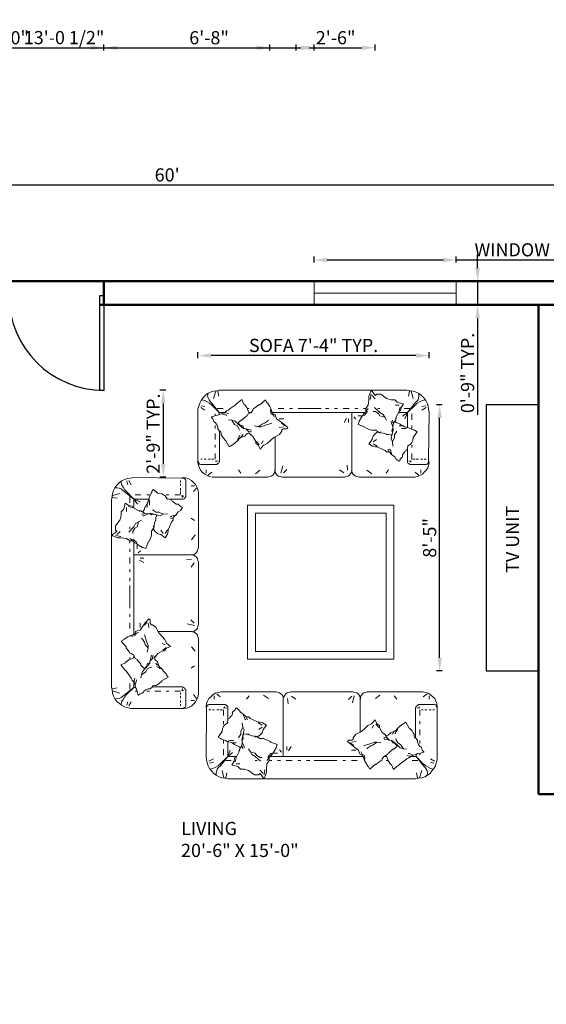
# Model space of a CAD drawing. Units: inches. Extents: x -46 to 764, y -530 to 112.
# Tile 4 of 5: x 307 to 507, y -262 to 112. Entities that reach past the tile are written whole.
import ezdxf

# ---------------------------------------------------------------- set-up
doc = ezdxf.new("R2010")
doc.units = ezdxf.units.IN
for name, color, linetype, lineweight in [('A-ANNO-DIMS', 2, 'Continuous', 18), ('A-AREA-IDEN', 7, 'Continuous', 18), ('A-DOOR', 3, 'Continuous', 25), ('A-FLOR-CASE', 32, 'Continuous', 25), ('A-GLAZ', 4, 'Continuous', 18), ('A-WALL', 7, 'Continuous', 50), ('furn', 28, 'Continuous', 18), ('txt', 167, 'Continuous', 18)]:
    doc.layers.add(name, color=color, linetype=linetype, lineweight=lineweight)
doc.styles.get("Standard").update_dxf_attribs({"font": 'arial.ttf'})
doc.dimstyles.new('ISO-25', dxfattribs={"dimtxt": 5, "dimasz": 5, "dimexe": 1.25, "dimexo": 0.625, "dimtad": 1, "dimlunit": 3, "dimtxsty": 'Standard', "dimcen": 2.5, "dimadec": 0, "dimazin": 0, "dimtfac": 1, "dimtmove": 0, "dimatfit": 3, "dimfxl": 1, "dimfxlon": 1, "dimarcsym": 0})

# ---------------------------------------------------------------- blocks, each defined once
blk = doc.blocks.new('*U2')
for p, q in [((0, 0), (0, -6)), ((40, 0), (40, -6))]:
    blk.add_line(p, q)
blk.add_lwpolyline([(0, 0), (0, 40), (1.75, 40), (1.75, 0)], close=True)
blk.add_arc((0, 0), 40, 0, 90)
blk = doc.blocks.new('sofa-36')
at = {"color": 0, "linetype": 'ByBlock'}
for p, q in [((-0.215, 0.805), (-0.2, 0.83)), ((-0.2, 0.83), (-0.215, 0.805)), ((-0.2, 0.83), (-0.18, 0.85)), ((-0.18, 0.85), (-0.2, 0.83)), ((-0.18, 0.85), (-0.16, 0.87)), ((-0.16, 0.87), (-0.18, 0.85)), ((-0.16, 0.87), (-0.135, 0.885)), ((-0.135, 0.885), (-0.16, 0.87)), ((-0.145, 0.825), (-0.145, 0.86)), ((-0.135, 0.885), (-0.105, 0.895)), ((-0.105, 0.895), (-0.135, 0.885)), ((-0.085, 0.85), (-0.12, 0.88)), ((-0.105, 0.895), (-0.08, 0.9)), ((-0.08, 0.9), (-0.105, 0.895)), ((-0.08, 0.9), (0.495, 0.9)), ((0.495, 0.9), (-0.08, 0.9)), ((0.19, 0.825), (0.215, 0.86)), ((0.415, 0.83), (0.365, 0.865)), ((0.495, 0.9), (0.515, 0.895)), ((0.515, 0.895), (0.495, 0.9)), ((0.515, 0.895), (0.53, 0.89)), ((0.53, 0.89), (0.515, 0.895)), ((0.53, 0.89), (0.545, 0.88)), ((0.545, 0.88), (0.53, 0.89)), ((0.545, 0.88), (0.56, 0.865)), ((0.56, 0.865), (0.545, 0.88)), ((0.56, 0.865), (0.57, 0.85)), ((0.57, 0.85), (0.56, 0.865)), ((0.57, 0.83), (0.575, 0.85)), ((0.57, 0.85), (0.57, 0.83)), ((0.57, 0.83), (0.57, 0.85)), ((0.57, 0.83), (0.575, 0.85)), ((0.57, 0.835), (0.57, 0.23)), ((0.57, 0.815), (0.57, 0.83)), ((0.57, 0.815), (0.57, 0.83)), ((0.575, 0.85), (0.585, 0.865)), ((0.575, 0.85), (0.585, 0.865)), ((0.585, 0.865), (0.595, 0.88)), ((0.585, 0.865), (0.595, 0.88)), ((0.595, 0.88), (0.61, 0.89)), ((0.595, 0.88), (0.61, 0.89)), ((0.61, 0.89), (0.63, 0.895)), ((0.61, 0.89), (0.63, 0.895)), ((0.615, 0.83), (0.62, 0.775)), ((0.63, 0.895), (0.645, 0.9)), ((0.63, 0.895), (0.645, 0.9)), ((0.645, 0.9), (0.87, 0.9)), ((0.87, 0.9), (0.645, 0.9)), ((0.655, 0.855), (0.7, 0.825)), ((0.87, 0.9), (1.29, 0.9)), ((1.29, 0.9), (0.87, 0.9)), ((1.28, 0.855), (1.245, 0.82)), ((1.305, 0.86), (1.285, 0.785)), ((1.29, 0.9), (1.31, 0.895)), ((1.31, 0.895), (1.29, 0.9)), ((1.31, 0.895), (1.33, 0.89)), ((1.33, 0.89), (1.31, 0.895)), ((1.33, 0.89), (1.345, 0.88)), ((1.345, 0.88), (1.33, 0.89)), ((1.345, 0.88), (1.355, 0.865)), ((1.355, 0.865), (1.345, 0.88)), ((1.355, 0.865), (1.365, 0.85)), ((1.365, 0.85), (1.355, 0.865)), ((1.365, 0.85), (1.368, 0.84)), ((1.37, 0.83), (1.365, 0.85)), ((1.365, 0.83), (1.37, 0.85)), ((1.365, 0.835), (1.365, 0.48)), ((1.365, 0.815), (1.37, 0.83)), ((1.365, 0.815), (1.365, 0.83)), ((1.368, 0.84), (1.37, 0.85)), ((1.37, 0.85), (1.38, 0.865)), ((1.37, 0.85), (1.38, 0.865)), ((1.38, 0.865), (1.39, 0.88)), ((1.38, 0.865), (1.39, 0.88)), ((1.39, 0.88), (1.405, 0.89)), ((1.39, 0.88), (1.405, 0.89)), ((1.405, 0.89), (1.425, 0.895)), ((1.405, 0.89), (1.425, 0.895)), ((1.425, 0.895), (1.44, 0.9)), ((1.425, 0.895), (1.44, 0.9)), ((1.44, 0.9), (2.015, 0.9)), ((2.015, 0.9), (1.44, 0.9)), ((1.525, 0.83), (1.57, 0.865)), ((1.745, 0.825), (1.72, 0.86)), ((2.015, 0.9), (2.045, 0.895)), ((2.045, 0.895), (2.015, 0.9)), ((2.02, 0.85), (2.06, 0.88)), ((2.045, 0.895), (2.07, 0.885)), ((2.07, 0.885), (2.045, 0.895)), ((2.07, 0.885), (2.095, 0.87)), ((2.095, 0.87), (2.07, 0.885)), ((2.08, 0.825), (2.08, 0.86)), ((2.095, 0.87), (2.12, 0.85)), ((2.12, 0.85), (2.095, 0.87)), ((2.12, 0.85), (2.14, 0.83)), ((2.14, 0.83), (2.12, 0.85)), ((2.14, 0.83), (2.15, 0.805)), ((2.15, 0.805), (2.14, 0.83)), ((-0.23, 0.75), (-0.225, 0.78)), ((-0.225, 0.78), (-0.23, 0.75)), ((-0.225, 0.72), (-0.23, 0.75)), ((-0.23, 0.75), (-0.225, 0.72)), ((-0.23, 0.23), (-0.225, 0.72)), ((-0.23, 0.23), (-0.225, 0.72)), ((-0.225, 0.78), (-0.215, 0.805)), ((-0.215, 0.805), (-0.225, 0.78)), ((-0.225, 0.745), (-0.22, 0.755)), ((-0.225, 0.735), (-0.225, 0.745)), ((-0.225, 0.72), (-0.225, 0.735)), ((-0.22, 0.755), (-0.21, 0.765)), ((-0.21, 0.765), (-0.2, 0.77)), ((-0.2, 0.77), (-0.19, 0.77)), ((-0.2, 0.715), (-0.18, 0.715)), ((-0.19, 0.77), (-0.175, 0.77)), ((-0.175, 0.77), (-0.055, 0.77)), ((-0.165, 0.715), (-0.145, 0.715)), ((-0.12, 0.715), (-0.095, 0.715)), ((-0.085, 0.715), (-0.06, 0.715)), ((-0.055, 0.77), (-0.04, 0.77)), ((-0.05, 0.715), (-0.05, 0.655)), ((-0.045, 0.735), (-0.035, 0.745)), ((-0.045, 0.73), (-0.02, 0.735)), ((-0.04, 0.77), (-0.03, 0.77)), ((-0.03, 0.77), (-0.02, 0.76)), ((-0.02, 0.76), (-0.01, 0.755)), ((-0.01, 0.755), (-0.005, 0.745)), ((-0.005, 0.745), (-0.005, 0.735)), ((-0.005, 0.735), (-0.005, 0.72)), ((-0.005, 0.72), (-0.005, 0.6)), ((0.07, 0.715), (0.045, 0.69)), ((0.075, 0.73), (0.07, 0.715)), ((0.08, 0.735), (0.075, 0.73)), ((0.11, 0.715), (0.08, 0.735)), ((0.125, 0.69), (0.11, 0.715)), ((1.94, 0.735), (1.945, 0.745)), ((1.94, 0.72), (1.94, 0.735)), ((1.94, 0.42), (1.94, 0.72)), ((1.945, 0.745), (1.95, 0.755)), ((1.95, 0.755), (1.96, 0.76)), ((1.98, 0.73), (1.955, 0.735)), ((1.96, 0.76), (1.97, 0.77)), ((1.97, 0.77), (1.98, 0.77)), ((1.98, 0.735), (1.975, 0.745)), ((1.98, 0.77), (1.99, 0.77)), ((1.985, 0.715), (1.985, 0.655)), ((1.99, 0.77), (2.115, 0.77)), ((2.02, 0.715), (2, 0.715)), ((2.055, 0.715), (2.035, 0.715)), ((2.1, 0.715), (2.08, 0.715)), ((2.115, 0.77), (2.125, 0.77)), ((2.135, 0.715), (2.12, 0.715)), ((2.125, 0.77), (2.135, 0.77)), ((2.135, 0.77), (2.15, 0.765)), ((2.15, 0.805), (2.16, 0.78)), ((2.16, 0.78), (2.15, 0.805)), ((2.15, 0.765), (2.155, 0.755)), ((2.155, 0.755), (2.16, 0.745)), ((2.16, 0.78), (2.165, 0.75)), ((2.165, 0.75), (2.16, 0.78)), ((2.16, 0.745), (2.165, 0.735)), ((2.165, 0.75), (2.165, 0.72)), ((2.165, 0.72), (2.165, 0.75)), ((2.165, 0.735), (2.165, 0.72)), ((2.165, 0.72), (2.165, 0.23)), ((2.165, 0.72), (2.165, 0.23)), ((0, 0.62), (-0.01, 0.585)), ((0.02, 0.63), (0, 0.62)), ((0.035, 0.655), (0.02, 0.64)), ((0.02, 0.64), (0.02, 0.63)), ((0.045, 0.67), (0.035, 0.655)), ((0.045, 0.69), (0.045, 0.68)), ((0.045, 0.68), (0.045, 0.67)), ((0.14, 0.68), (0.125, 0.69)), ((0.155, 0.67), (0.14, 0.68)), ((0.155, 0.67), (0.17, 0.62)), ((0.185, 0.64), (0.155, 0.67)), ((0.17, 0.62), (0.18, 0.61)), ((0.185, 0.64), (0.21, 0.64)), ((0.19, 0.64), (0.185, 0.64)), ((0.195, 0.61), (0.19, 0.64)), ((0.21, 0.64), (0.225, 0.625)), ((0.225, 0.625), (0.25, 0.615)), ((0.235, 0.62), (0.235, 0.62)), ((0.25, 0.615), (0.31, 0.585)), ((-0.06, 0.52), (-0.065, 0.49)), ((-0.05, 0.54), (-0.06, 0.52)), ((-0.05, 0.595), (-0.05, 0.565)), ((-0.04, 0.555), (-0.05, 0.54)), ((-0.025, 0.565), (-0.04, 0.555)), ((-0.005, 0.58), (-0.025, 0.565)), ((-0.01, 0.585), (-0.005, 0.58)), ((0.15, 0.535), (0.13, 0.49)), ((0.15, 0.535), (0.145, 0.58)), ((0.165, 0.505), (0.15, 0.535)), ((0.31, 0.585), (0.325, 0.585)), ((0.35, 0.555), (0.31, 0.58)), ((0.35, 0.535), (0.315, 0.51)), ((0.325, 0.585), (0.355, 0.58)), ((0.355, 0.58), (0.395, 0.555)), ((0.395, 0.555), (0.36, 0.51)), ((1.415, 0.52), (1.38, 0.49)), ((1.445, 0.55), (1.415, 0.52)), ((1.475, 0.565), (1.445, 0.55)), ((1.485, 0.57), (1.475, 0.565)), ((1.52, 0.61), (1.485, 0.57)), ((1.505, 0.555), (1.49, 0.525)), ((1.54, 0.57), (1.52, 0.61)), ((1.53, 0.565), (1.56, 0.53)), ((1.565, 0.55), (1.54, 0.57)), ((1.565, 0.53), (1.565, 0.55)), ((1.595, 0.48), (1.565, 0.53)), ((1.735, 0.5), (1.755, 0.525)), ((1.755, 0.525), (1.75, 0.5)), ((1.755, 0.525), (1.775, 0.54)), ((1.775, 0.54), (1.805, 0.565)), ((1.805, 0.565), (1.815, 0.57)), ((1.815, 0.57), (1.84, 0.585)), ((1.84, 0.585), (1.875, 0.525)), ((1.875, 0.525), (1.88, 0.52)), ((1.88, 0.52), (1.905, 0.495)), ((1.985, 0.595), (1.985, 0.565)), ((-0.07, 0.48), (-0.105, 0.43)), ((-0.105, 0.43), (-0.08, 0.415)), ((-0.08, 0.415), (-0.07, 0.41)), ((-0.065, 0.49), (-0.07, 0.48)), ((-0.07, 0.41), (-0.03, 0.395)), ((0.115, 0.44), (0.105, 0.425)), ((0.13, 0.46), (0.115, 0.44)), ((0.13, 0.49), (0.13, 0.46)), ((0.14, 0.4), (0.155, 0.465)), ((0.155, 0.415), (0.145, 0.4)), ((0.16, 0.465), (0.15, 0.44)), ((0.15, 0.44), (0.155, 0.415)), ((0.155, 0.465), (0.165, 0.505)), ((0.165, 0.465), (0.16, 0.465)), ((0.185, 0.46), (0.165, 0.465)), ((0.21, 0.46), (0.185, 0.46)), ((0.215, 0.455), (0.21, 0.46)), ((0.23, 0.45), (0.215, 0.455)), ((0.245, 0.445), (0.23, 0.45)), ((0.275, 0.44), (0.245, 0.445)), ((0.275, 0.43), (0.275, 0.44)), ((0.285, 0.44), (0.275, 0.43)), ((0.325, 0.415), (0.285, 0.44)), ((0.325, 0.45), (0.3, 0.43)), ((0.32, 0.415), (0.325, 0.415)), ((0.355, 0.415), (0.32, 0.415)), ((0.35, 0.475), (0.325, 0.45)), ((0.36, 0.505), (0.35, 0.475)), ((0.365, 0.415), (0.355, 0.415)), ((0.36, 0.51), (0.36, 0.505)), ((0.38, 0.41), (0.365, 0.415)), ((0.405, 0.4), (0.38, 0.41)), ((1.295, 0.41), (1.28, 0.4)), ((1.32, 0.46), (1.295, 0.425)), ((1.295, 0.425), (1.295, 0.41)), ((1.38, 0.49), (1.32, 0.46)), ((1.62, 0.46), (1.595, 0.48)), ((1.615, 0.46), (1.61, 0.46)), ((1.61, 0.43), (1.635, 0.425)), ((1.62, 0.41), (1.61, 0.415)), ((1.63, 0.45), (1.62, 0.46)), ((1.67, 0.4), (1.62, 0.41)), ((1.655, 0.45), (1.625, 0.445)), ((1.645, 0.425), (1.63, 0.45)), ((1.635, 0.425), (1.645, 0.425)), ((1.645, 0.425), (1.67, 0.4)), ((1.68, 0.475), (1.655, 0.45)), ((1.69, 0.48), (1.68, 0.475)), ((1.72, 0.49), (1.69, 0.48)), ((1.695, 0.46), (1.705, 0.465)), ((1.705, 0.465), (1.72, 0.49)), ((1.72, 0.49), (1.735, 0.5)), ((1.74, 0.49), (1.73, 0.465)), ((1.74, 0.4), (1.735, 0.415)), ((1.75, 0.5), (1.74, 0.49)), ((1.905, 0.495), (1.915, 0.475)), ((1.915, 0.475), (1.925, 0.46)), ((1.925, 0.46), (1.925, 0.45)), ((1.925, 0.45), (1.93, 0.425)), ((1.93, 0.425), (1.94, 0.425)), ((1.94, 0.425), (1.96, 0.4)), ((1.985, 0.45), (1.985, 0.51)), ((-0.05, 0.365), (-0.05, 0.395)), ((-0.03, 0.395), (-0.01, 0.385)), ((-0.01, 0.385), (0.015, 0.395)), ((-0.01, 0.385), (0.02, 0.38)), ((-0.005, 0.385), (-0.005, 0.23)), ((0.015, 0.395), (0.03, 0.395)), ((0.02, 0.38), (0.04, 0.37)), ((0.03, 0.395), (0.055, 0.395)), ((0.04, 0.37), (0.065, 0.355)), ((0.04, 0.37), (0.065, 0.37)), ((0.065, 0.37), (0.08, 0.37)), ((0.065, 0.355), (0.07, 0.35)), ((0.07, 0.35), (0.11, 0.335)), ((0.11, 0.335), (0.13, 0.32)), ((0.125, 0.32), (0.115, 0.305)), ((0.14, 0.34), (0.125, 0.32)), ((0.145, 0.38), (0.14, 0.34)), ((0.14, 0.34), (0.145, 0.335)), ((0.145, 0.4), (0.145, 0.38)), ((0.145, 0.38), (0.165, 0.33)), ((0.145, 0.335), (0.15, 0.31)), ((0.165, 0.33), (0.165, 0.32)), ((0.23, 0.28), (0.21, 0.31)), ((0.435, 0.385), (0.405, 0.4)), ((0.44, 0.38), (0.435, 0.385)), ((0.505, 0.355), (0.44, 0.38)), ((0.47, 0.28), (0.495, 0.32)), ((0.495, 0.325), (0.505, 0.355)), ((0.495, 0.32), (0.495, 0.325)), ((0.605, 0.295), (0.605, 0.335)), ((0.625, 0.29), (0.65, 0.335)), ((1.245, 0.4), (1.235, 0.385)), ((1.235, 0.385), (1.275, 0.35)), ((1.28, 0.4), (1.245, 0.4)), ((1.265, 0.37), (1.3, 0.34)), ((1.275, 0.35), (1.31, 0.325)), ((1.28, 0.38), (1.325, 0.385)), ((1.31, 0.325), (1.35, 0.295)), ((1.4, 0.34), (1.475, 0.365)), ((1.445, 0.32), (1.435, 0.31)), ((1.475, 0.34), (1.445, 0.32)), ((1.475, 0.365), (1.51, 0.38)), ((1.5, 0.35), (1.475, 0.34)), ((1.54, 0.38), (1.5, 0.35)), ((1.51, 0.38), (1.54, 0.38)), ((1.54, 0.38), (1.58, 0.37)), ((1.67, 0.4), (1.69, 0.395)), ((1.69, 0.4), (1.75, 0.35)), ((1.69, 0.395), (1.7, 0.37)), ((1.7, 0.37), (1.72, 0.37)), ((1.735, 0.325), (1.715, 0.305)), ((1.72, 0.37), (1.75, 0.34)), ((1.745, 0.335), (1.735, 0.325)), ((1.755, 0.37), (1.74, 0.4)), ((1.75, 0.34), (1.745, 0.335)), ((1.75, 0.35), (1.78, 0.32)), ((1.785, 0.355), (1.755, 0.37)), ((1.78, 0.32), (1.815, 0.31)), ((1.815, 0.31), (1.785, 0.355)), ((1.815, 0.31), (1.85, 0.305)), ((1.96, 0.4), (1.96, 0.38)), ((1.96, 0.38), (1.965, 0.37)), ((1.965, 0.37), (1.97, 0.355)), ((1.97, 0.355), (1.985, 0.335)), ((1.985, 0.365), (1.985, 0.395)), ((1.985, 0.335), (1.995, 0.33)), ((1.995, 0.33), (2, 0.325)), ((2, 0.325), (2.01, 0.295)), ((-0.225, 0.195), (-0.23, 0.23)), ((-0.225, 0.195), (-0.23, 0.23)), ((-0.2, 0.18), (-0.155, 0.205)), ((-0.005, 0.23), (-0.085, 0.13)), ((-0.005, 0.23), (-0.085, 0.155)), ((-0.05, 0.245), (-0.05, 0.305)), ((0.02, 0.295), (-0.005, 0.23)), ((0.045, 0.27), (-0.005, 0.23)), ((0.085, 0.23), (-0.005, 0.23)), ((0.065, 0.215), (0.06, 0.18)), ((0.08, 0.22), (0.065, 0.215)), ((0.07, 0.175), (0.08, 0.215)), ((0.11, 0.275), (0.08, 0.22)), ((0.115, 0.305), (0.11, 0.275)), ((0.12, 0.295), (0.115, 0.29)), ((0.23, 0.28), (0.28, 0.265)), ((0.245, 0.25), (0.23, 0.28)), ((0.28, 0.23), (0.245, 0.25)), ((0.28, 0.265), (0.295, 0.24)), ((0.335, 0.18), (0.28, 0.23)), ((0.295, 0.24), (0.33, 0.22)), ((0.33, 0.22), (0.35, 0.22)), ((0.41, 0.22), (0.425, 0.24)), ((0.425, 0.22), (0.41, 0.2)), ((0.425, 0.24), (0.44, 0.26)), ((0.425, 0.22), (0.445, 0.24)), ((0.425, 0.19), (0.425, 0.22)), ((0.435, 0.23), (0.87, 0.23)), ((0.44, 0.26), (0.46, 0.265)), ((0.445, 0.24), (0.46, 0.265)), ((0.46, 0.265), (0.47, 0.28)), ((0.51, 0.265), (0.47, 0.265)), ((0.55, 0.275), (0.53, 0.3)), ((1.395, 0.23), (0.87, 0.23)), ((1.325, 0.295), (1.275, 0.295)), ((1.35, 0.295), (1.36, 0.265)), ((1.36, 0.265), (1.365, 0.25)), ((1.365, 0.25), (1.395, 0.24)), ((1.38, 0.265), (1.375, 0.28)), ((1.395, 0.24), (1.38, 0.265)), ((1.4, 0.22), (1.395, 0.24)), ((1.41, 0.19), (1.4, 0.22)), ((1.41, 0.23), (1.405, 0.25)), ((1.415, 0.215), (1.41, 0.23)), ((1.41, 0.19), (1.415, 0.215)), ((1.595, 0.205), (1.59, 0.19)), ((1.615, 0.235), (1.595, 0.205)), ((1.65, 0.25), (1.615, 0.23)), ((1.615, 0.23), (1.615, 0.235)), ((1.615, 0.23), (1.615, 0.23)), ((1.64, 0.23), (1.62, 0.23)), ((1.645, 0.215), (1.635, 0.24)), ((1.66, 0.18), (1.645, 0.215)), ((1.655, 0.265), (1.65, 0.25)), ((1.66, 0.265), (1.655, 0.265)), ((1.675, 0.28), (1.66, 0.265)), ((1.695, 0.295), (1.675, 0.28)), ((1.705, 0.305), (1.695, 0.295)), ((1.715, 0.305), (1.705, 0.305)), ((1.85, 0.205), (1.83, 0.19)), ((1.88, 0.235), (1.85, 0.24)), ((1.87, 0.215), (1.85, 0.205)), ((1.875, 0.26), (1.865, 0.26)), ((1.89, 0.235), (1.87, 0.215)), ((1.87, 0.215), (1.88, 0.22)), ((1.92, 0.245), (1.875, 0.26)), ((1.89, 0.235), (1.88, 0.235)), ((1.885, 0.23), (1.945, 0.23)), ((1.92, 0.245), (1.89, 0.235)), ((1.945, 0.25), (1.92, 0.245)), ((1.96, 0.26), (1.945, 0.25)), ((1.945, 0.25), (1.945, 0.23)), ((1.945, 0.23), (2.025, 0.13)), ((1.945, 0.23), (2.02, 0.155)), ((1.99, 0.265), (1.96, 0.26)), ((1.985, 0.245), (1.985, 0.26)), ((2.025, 0.275), (1.99, 0.265)), ((2.01, 0.295), (2.025, 0.28)), ((2.025, 0.28), (2.025, 0.275)), ((2.135, 0.18), (2.095, 0.205)), ((2.165, 0.23), (2.165, 0.195)), ((2.165, 0.23), (2.165, 0.195)), ((-0.22, 0.165), (-0.225, 0.195)), ((-0.22, 0.165), (-0.225, 0.195)), ((-0.21, 0.135), (-0.22, 0.165)), ((-0.21, 0.135), (-0.22, 0.165)), ((-0.195, 0.105), (-0.21, 0.135)), ((-0.195, 0.105), (-0.21, 0.135)), ((-0.155, 0.17), (-0.195, 0.16)), ((-0.175, 0.08), (-0.195, 0.105)), ((-0.175, 0.08), (-0.195, 0.105)), ((-0.16, 0.105), (-0.185, 0.1)), ((-0.13, 0.12), (-0.16, 0.105)), ((-0.105, 0.135), (-0.13, 0.12)), ((-0.1, 0.115), (-0.115, 0.1)), ((-0.085, 0.155), (-0.105, 0.135)), ((-0.085, 0.13), (-0.1, 0.115)), ((-0.03, 0.19), (0.03, 0.19)), ((0.06, 0.18), (0.035, 0.14)), ((0.035, 0.14), (0.085, 0.13)), ((0.08, 0.155), (0.12, 0.155)), ((0.085, 0.13), (0.1, 0.125)), ((0.1, 0.125), (0.125, 0.1)), ((0.28, 0.19), (0.3, 0.19)), ((0.395, 0.1), (0.4, 0.155)), ((0.41, 0.2), (0.4, 0.19)), ((0.4, 0.155), (0.42, 0.18)), ((0.42, 0.18), (0.425, 0.19)), ((0.45, 0.19), (0.425, 0.19)), ((0.54, 0.19), (0.51, 0.19)), ((0.6, 0.19), (0.66, 0.19)), ((0.72, 0.19), (0.75, 0.19)), ((0.81, 0.19), (0.845, 0.19)), ((1.125, 0.19), (0.89, 0.19)), ((1.215, 0.19), (1.185, 0.19)), ((1.335, 0.19), (1.275, 0.19)), ((1.42, 0.17), (1.41, 0.19)), ((1.445, 0.13), (1.42, 0.17)), ((1.45, 0.13), (1.445, 0.13)), ((1.465, 0.1), (1.45, 0.13)), ((1.525, 0.15), (1.465, 0.1)), ((1.535, 0.15), (1.525, 0.15)), ((1.56, 0.17), (1.535, 0.15)), ((1.58, 0.185), (1.56, 0.17)), ((1.59, 0.19), (1.58, 0.185)), ((1.655, 0.19), (1.635, 0.19)), ((1.68, 0.15), (1.66, 0.18)), ((1.69, 0.145), (1.68, 0.15)), ((1.71, 0.095), (1.69, 0.145)), ((1.745, 0.125), (1.71, 0.095)), ((1.765, 0.14), (1.745, 0.125)), ((1.78, 0.155), (1.765, 0.14)), ((1.83, 0.19), (1.78, 0.155)), ((1.845, 0.2), (1.845, 0.2)), ((1.965, 0.19), (1.905, 0.19)), ((2.02, 0.155), (2.045, 0.135)), ((2.025, 0.13), (2.04, 0.115)), ((2.04, 0.115), (2.05, 0.1)), ((2.045, 0.135), (2.07, 0.12)), ((2.07, 0.12), (2.095, 0.105)), ((2.095, 0.17), (2.13, 0.16)), ((2.095, 0.105), (2.125, 0.1)), ((2.13, 0.105), (2.11, 0.08)), ((2.13, 0.105), (2.11, 0.08)), ((2.145, 0.135), (2.13, 0.105)), ((2.145, 0.135), (2.13, 0.105)), ((2.155, 0.165), (2.145, 0.135)), ((2.155, 0.165), (2.145, 0.135)), ((2.165, 0.195), (2.155, 0.165)), ((2.165, 0.195), (2.155, 0.165)), ((-0.15, 0.055), (-0.175, 0.08)), ((-0.15, 0.055), (-0.175, 0.08)), ((-0.125, 0.035), (-0.15, 0.055)), ((-0.125, 0.035), (-0.15, 0.055)), ((-0.12, 0.08), (-0.125, 0.06)), ((-0.125, 0.06), (-0.125, 0.035)), ((-0.095, 0.02), (-0.125, 0.035)), ((-0.095, 0.02), (-0.125, 0.035)), ((-0.115, 0.1), (-0.12, 0.08)), ((-0.065, 0.01), (-0.095, 0.02)), ((-0.065, 0.01), (-0.095, 0.02)), ((-0.045, 0.01), (-0.065, 0.085)), ((-0.035, 0.005), (-0.065, 0.01)), ((-0.035, 0.005), (-0.065, 0.01)), ((0, 0), (-0.035, 0.005)), ((0, 0), (-0.035, 0.005)), ((-0.015, 0.06), (-0.025, 0.01)), ((1.94, 0), (0, 0)), ((1.94, 0), (0, 0)), ((0.125, 0.1), (0.165, 0.1)), ((0.165, 0.1), (0.21, 0.085)), ((0.21, 0.085), (0.27, 0.04)), ((0.27, 0.04), (0.315, 0.04)), ((0.315, 0.04), (0.325, 0.055)), ((0.325, 0.055), (0.34, 0.04)), ((0.36, 0.055), (0.33, 0.09)), ((0.34, 0.04), (0.36, 0.01)), ((0.36, 0.01), (0.375, 0.01)), ((0.37, 0.04), (0.38, 0.095)), ((0.375, 0.01), (0.395, 0.065)), ((0.395, 0.065), (0.395, 0.1)), ((1.97, 0.005), (1.94, 0)), ((1.97, 0.005), (1.94, 0)), ((1.95, 0.06), (1.96, 0.01)), ((2.005, 0.01), (1.97, 0.005)), ((2.005, 0.01), (1.97, 0.005)), ((1.98, 0.01), (2.005, 0.085)), ((2.035, 0.02), (2.005, 0.01)), ((2.035, 0.02), (2.005, 0.01)), ((2.065, 0.035), (2.035, 0.02)), ((2.065, 0.035), (2.035, 0.02)), ((2.05, 0.1), (2.06, 0.08)), ((2.06, 0.08), (2.065, 0.06)), ((2.065, 0.06), (2.06, 0.035)), ((2.09, 0.055), (2.065, 0.035)), ((2.09, 0.055), (2.065, 0.035)), ((2.11, 0.08), (2.09, 0.055)), ((2.11, 0.08), (2.09, 0.055))]:
    blk.add_line(p, q, dxfattribs=at)
blk = doc.blocks.new('*D10')
at = {"layer": 'A-ANNO-DIMS', "color": 0, "lineweight": -2, "transparency": 16777216}
for p, q in [((2.62, 48.57), (2.62, 50.82)), ((7.62, 49.57), (717.62, 49.57)), ((722.62, 48.57), (722.62, 50.82))]:
    blk.add_line(p, q, dxfattribs=at)
at = {"layer": 'A-ANNO-DIMS', "color": 0, "transparency": 16777216}
for points in [[(7.62, 50.4), (7.62, 48.73), (2.62, 49.57)], [(717.62, 50.4), (717.62, 48.73), (722.62, 49.57)]]:
    blk.add_solid(points, dxfattribs=at)
at = {"layer": 'Defpoints', "color": 0, "transparency": 16777216}
for p in [(722.62, 49.57), (2.62, 12.97), (722.62, 12.97)]:
    blk.add_point(p, dxfattribs=at)
at = {"layer": 'A-ANNO-DIMS', "color": 0, "transparency": 16777216, "insert": (362.62, 52.74), "char_height": 5, "attachment_point": 5}
blk.add_mtext("60'", dxfattribs=at)
blk = doc.blocks.new('WIN-54IN')
blk.add_line((4.5, 54), (4.5, 0))
blk.add_lwpolyline([(0, 54), (9, 54), (9, 0), (0, 0)], close=True)
blk = doc.blocks.new('*D19')
at = {"layer": 'A-ANNO-DIMS', "color": 0, "lineweight": -2, "transparency": 16777216}
for p, q in [((418.45, 20.07), (418.45, 22.32)), ((423.45, 21.07), (467.45, 21.07)), ((472.45, 20.07), (472.45, 22.32)), ((472.45, 21.07), (541.97, 21.07))]:
    blk.add_line(p, q, dxfattribs=at)
at = {"layer": 'A-ANNO-DIMS', "color": 0, "transparency": 16777216}
for points in [[(423.45, 21.9), (423.45, 20.24), (418.45, 21.07)], [(467.45, 21.9), (467.45, 20.24), (472.45, 21.07)]]:
    blk.add_solid(points, dxfattribs=at)
at = {"layer": 'Defpoints', "color": 0, "transparency": 16777216}
for p in [(472.45, 21.07), (418.45, 12.97), (472.45, 12.97)]:
    blk.add_point(p, dxfattribs=at)
at = {"layer": 'A-ANNO-DIMS', "color": 0, "transparency": 16777216, "insert": (509.71, 24.28), "char_height": 5, "attachment_point": 5}
blk.add_mtext('WINDOW 4\'-6" TYP.', dxfattribs=at)
blk = doc.blocks.new('*D20')
at = {"layer": 'A-ANNO-DIMS', "color": 0, "lineweight": -2, "transparency": 16777216}
for p, q in [((480.55, 17.97), (480.55, 22.97)), ((479.55, 12.97), (481.8, 12.97)), ((480.55, 12.97), (480.55, 3.97)), ((479.55, 3.97), (481.8, 3.97)), ((480.55, -1.03), (480.55, -37.76))]:
    blk.add_line(p, q, dxfattribs=at)
at = {"layer": 'A-ANNO-DIMS', "color": 0, "transparency": 16777216}
for points in [[(479.71, 17.97), (481.38, 17.97), (480.55, 12.97)], [(479.71, -1.03), (481.38, -1.03), (480.55, 3.97)]]:
    blk.add_solid(points, dxfattribs=at)
at = {"layer": 'Defpoints', "color": 0, "transparency": 16777216}
for p in [(472.45, 12.97), (472.45, 3.97), (480.55, 3.97)]:
    blk.add_point(p, dxfattribs=at)
at = {"layer": 'A-ANNO-DIMS', "color": 0, "transparency": 16777216, "insert": (477.37, -21.89), "char_height": 5, "attachment_point": 5, "rotation": 90}
blk.add_mtext('0\'-9" TYP.', dxfattribs=at)
blk = doc.blocks.new('*D25')
at = {"layer": 'A-ANNO-DIMS', "color": 0, "lineweight": -2, "transparency": 16777216}
for p, q in [((374.31, -16.28), (374.31, -14.03)), ((462.12, -16.28), (462.12, -14.03)), ((457.12, -15.28), (379.31, -15.28))]:
    blk.add_line(p, q, dxfattribs=at)
at = {"layer": 'A-ANNO-DIMS', "color": 0, "transparency": 16777216}
for points in [[(379.31, -14.45), (379.31, -16.12), (374.31, -15.28)], [(457.12, -14.45), (457.12, -16.12), (462.12, -15.28)]]:
    blk.add_solid(points, dxfattribs=at)
at = {"layer": 'Defpoints', "color": 0, "transparency": 16777216}
for p in [(374.31, -15.28), (374.31, -28.45), (462.12, -28.45)]:
    blk.add_point(p, dxfattribs=at)
at = {"layer": 'A-ANNO-DIMS', "color": 0, "transparency": 16777216, "insert": (418.22, -12.07), "char_height": 5, "attachment_point": 5}
blk.add_mtext('SOFA 7\'-4" TYP.', dxfattribs=at)
blk = doc.blocks.new('*D26')
at = {"layer": 'A-ANNO-DIMS', "color": 0, "lineweight": -2, "transparency": 16777216}
for p, q in [((362.14, -28.45), (359.89, -28.45)), ((361.14, -33.45), (361.14, -56.45)), ((362.14, -61.45), (359.89, -61.45))]:
    blk.add_line(p, q, dxfattribs=at)
at = {"layer": 'A-ANNO-DIMS', "color": 0, "transparency": 16777216}
for points in [[(360.31, -33.45), (361.97, -33.45), (361.14, -28.45)], [(360.31, -56.45), (361.97, -56.45), (361.14, -61.45)]]:
    blk.add_solid(points, dxfattribs=at)
at = {"layer": 'Defpoints', "color": 0, "transparency": 16777216}
for p in [(374.31, -28.45), (361.14, -61.45), (374.31, -61.45)]:
    blk.add_point(p, dxfattribs=at)
at = {"layer": 'A-ANNO-DIMS', "color": 0, "transparency": 16777216, "insert": (357.96, -44.95), "char_height": 5, "attachment_point": 5, "rotation": 90}
blk.add_mtext('2\'-9" TYP.', dxfattribs=at)
blk = doc.blocks.new('*D39')
at = {"layer": 'A-ANNO-DIMS', "color": 0, "lineweight": -2, "transparency": 16777216}
for p, q in [((467.12, -33.96), (464.87, -33.96)), ((466.12, -130.15), (466.12, -38.96)), ((467.12, -135.15), (464.87, -135.15))]:
    blk.add_line(p, q, dxfattribs=at)
at = {"layer": 'A-ANNO-DIMS', "color": 0, "transparency": 16777216}
for points in [[(465.29, -38.96), (466.96, -38.96), (466.12, -33.96)], [(465.29, -130.15), (466.96, -130.15), (466.12, -135.15)]]:
    blk.add_solid(points, dxfattribs=at)
at = {"layer": 'Defpoints', "color": 0, "transparency": 16777216}
for p in [(466.12, -33.96), (503.62, -33.96), (503.62, -135.15)]:
    blk.add_point(p, dxfattribs=at)
at = {"layer": 'A-ANNO-DIMS', "color": 0, "transparency": 16777216, "insert": (462.95, -84.56), "char_height": 5, "attachment_point": 5, "rotation": 90}
blk.add_mtext('8\'-5"', dxfattribs=at)
blk = doc.blocks.new('*D40')
at = {"layer": 'A-ANNO-DIMS', "color": 0, "lineweight": -2, "transparency": 16777216}
for p, q in [((483.74, -503.53), (483.74, -505.78)), ((488.74, -504.53), (498.62, -504.53)), ((503.62, -503.53), (503.62, -505.78))]:
    blk.add_line(p, q, dxfattribs=at)
at = {"layer": 'A-ANNO-DIMS', "color": 0, "transparency": 16777216}
for points in [[(488.74, -503.7), (488.74, -505.36), (483.74, -504.53)], [(498.62, -503.7), (498.62, -505.36), (503.62, -504.53)]]:
    blk.add_solid(points, dxfattribs=at)
at = {"layer": 'Defpoints', "color": 0, "transparency": 16777216}
for p in [(483.74, -135.15), (503.62, -135.15), (503.62, -504.53)]:
    blk.add_point(p, dxfattribs=at)
at = {"layer": 'A-ANNO-DIMS', "color": 0, "transparency": 16777216, "insert": (493.68, -501.35), "char_height": 5, "attachment_point": 5}
blk.add_mtext('1\'-8"', dxfattribs=at)
blk = doc.blocks.new('*D41')
at = {"layer": 'A-ANNO-DIMS', "color": 0, "lineweight": -2, "transparency": 16777216}
for p, q in [((393.18, -503.53), (393.18, -505.78)), ((398.18, -504.53), (443.74, -504.53)), ((448.74, -503.53), (448.74, -505.78))]:
    blk.add_line(p, q, dxfattribs=at)
at = {"layer": 'A-ANNO-DIMS', "color": 0, "transparency": 16777216}
for points in [[(398.18, -503.7), (398.18, -505.36), (393.18, -504.53)], [(443.74, -503.7), (443.74, -505.36), (448.74, -504.53)]]:
    blk.add_solid(points, dxfattribs=at)
at = {"layer": 'Defpoints', "color": 0, "transparency": 16777216}
for p in [(393.18, -72.15), (448.74, -72.15), (448.74, -504.53)]:
    blk.add_point(p, dxfattribs=at)
at = {"layer": 'A-ANNO-DIMS', "color": 0, "transparency": 16777216, "insert": (420.96, -501.32), "char_height": 5, "attachment_point": 5}
blk.add_mtext('4\'-7 1/2"', dxfattribs=at)
blk = doc.blocks.new('*D42')
at = {"layer": 'A-ANNO-DIMS', "color": 0, "lineweight": -2, "transparency": 16777216}
for p, q in [((759.12, -72.15), (761.37, -72.15)), ((760.12, -77.15), (760.12, -125.72)), ((759.12, -130.72), (761.37, -130.72))]:
    blk.add_line(p, q, dxfattribs=at)
at = {"layer": 'A-ANNO-DIMS', "color": 0, "transparency": 16777216}
for points in [[(759.29, -77.15), (760.96, -77.15), (760.12, -72.15)], [(759.29, -125.72), (760.96, -125.72), (760.12, -130.72)]]:
    blk.add_solid(points, dxfattribs=at)
at = {"layer": 'Defpoints', "color": 0, "transparency": 16777216}
for p in [(448.74, -72.15), (448.74, -130.72), (760.12, -130.72)]:
    blk.add_point(p, dxfattribs=at)
at = {"layer": 'A-ANNO-DIMS', "color": 0, "transparency": 16777216, "insert": (756.91, -101.44), "char_height": 5, "attachment_point": 5, "rotation": 90}
blk.add_mtext('4\'-10 1/2"', dxfattribs=at)
blk = doc.blocks.new('*D48')
at = {"layer": 'A-ANNO-DIMS', "color": 0, "lineweight": -2, "transparency": 16777216}
for p, q in [((-33.88, 3.97), (-36.13, 3.97)), ((-34.88, -1.03), (-34.88, -51.03)), ((-33.88, -56.03), (-36.13, -56.03))]:
    blk.add_line(p, q, dxfattribs=at)
at = {"layer": 'A-ANNO-DIMS', "color": 0, "transparency": 16777216}
for points in [[(-35.71, -1.03), (-34.04, -1.03), (-34.88, 3.97)], [(-35.71, -51.03), (-34.04, -51.03), (-34.88, -56.03)]]:
    blk.add_solid(points, dxfattribs=at)
at = {"layer": 'Defpoints', "color": 0, "transparency": 16777216}
for p in [(713.62, 3.97), (-34.88, -56.03), (713.62, -56.03)]:
    blk.add_point(p, dxfattribs=at)
at = {"layer": 'A-ANNO-DIMS', "color": 0, "transparency": 16777216, "insert": (-38.05, -26.03), "char_height": 5, "attachment_point": 5, "rotation": 90}
blk.add_mtext('5\'-0"', dxfattribs=at)
blk = doc.blocks.new('*D51')
at = {"layer": 'A-ANNO-DIMS', "color": 0, "lineweight": -2, "transparency": 16777216}
for p, q in [((266.62, 100.72), (266.62, 102.97)), ((271.62, 101.72), (333.62, 101.72)), ((338.62, 100.72), (338.62, 102.97))]:
    blk.add_line(p, q, dxfattribs=at)
at = {"layer": 'A-ANNO-DIMS', "color": 0, "transparency": 16777216}
for points in [[(271.62, 102.55), (271.62, 100.88), (266.62, 101.72)], [(333.62, 102.55), (333.62, 100.88), (338.62, 101.72)]]:
    blk.add_solid(points, dxfattribs=at)
at = {"layer": 'Defpoints', "color": 0, "transparency": 16777216}
for p in [(338.62, 101.72), (266.62, 12.97), (338.62, 12.97)]:
    blk.add_point(p, dxfattribs=at)
at = {"layer": 'A-ANNO-DIMS', "color": 0, "transparency": 16777216, "insert": (302.62, 104.89), "char_height": 5, "attachment_point": 5}
blk.add_mtext('6\'-0"', dxfattribs=at)
blk = doc.blocks.new('*D52')
at = {"layer": 'A-ANNO-DIMS', "color": 0, "lineweight": -2, "transparency": 16777216}
for p, q in [((338.62, 100.72), (338.62, 102.97)), ((343.62, 101.72), (413.45, 101.72)), ((418.45, 100.72), (418.45, 102.97))]:
    blk.add_line(p, q, dxfattribs=at)
at = {"layer": 'A-ANNO-DIMS', "color": 0, "transparency": 16777216}
for points in [[(343.62, 102.55), (343.62, 100.88), (338.62, 101.72)], [(413.45, 102.55), (413.45, 100.88), (418.45, 101.72)]]:
    blk.add_solid(points, dxfattribs=at)
at = {"layer": 'Defpoints', "color": 0, "transparency": 16777216}
for p in [(418.45, 101.72), (338.62, 12.97), (418.45, 12.97)]:
    blk.add_point(p, dxfattribs=at)
at = {"layer": 'A-ANNO-DIMS', "color": 0, "transparency": 16777216, "insert": (378.54, 104.89), "char_height": 5, "attachment_point": 5}
blk.add_mtext('6\'-8"', dxfattribs=at)
blk = doc.blocks.new('*D76')
at = {"layer": 'A-ANNO-DIMS', "color": 0, "lineweight": -2, "transparency": 16777216}
for p, q in [((411.62, 100.72), (411.62, 102.97)), ((416.62, 101.72), (436.62, 101.72)), ((441.62, 100.72), (441.62, 102.97))]:
    blk.add_line(p, q, dxfattribs=at)
at = {"layer": 'A-ANNO-DIMS', "color": 0, "transparency": 16777216}
for points in [[(416.62, 102.55), (416.62, 100.88), (411.62, 101.72)], [(436.62, 102.55), (436.62, 100.88), (441.62, 101.72)]]:
    blk.add_solid(points, dxfattribs=at)
at = {"layer": 'Defpoints', "color": 0, "transparency": 16777216}
for p in [(441.62, 101.72), (411.62, -272.03), (441.62, -272.03)]:
    blk.add_point(p, dxfattribs=at)
at = {"layer": 'A-ANNO-DIMS', "color": 0, "transparency": 16777216, "insert": (426.62, 104.89), "char_height": 5, "attachment_point": 5}
blk.add_mtext('2\'-6"', dxfattribs=at)
blk = doc.blocks.new('*D78')
at = {"layer": 'A-ANNO-DIMS', "color": 0, "lineweight": -2, "transparency": 16777216}
for p, q in [((245.34, 100.72), (245.34, 102.97)), ((250.34, 101.72), (396.62, 101.72)), ((401.62, 100.72), (401.62, 102.97))]:
    blk.add_line(p, q, dxfattribs=at)
at = {"layer": 'A-ANNO-DIMS', "color": 0, "transparency": 16777216}
for points in [[(250.34, 102.55), (250.34, 100.88), (245.34, 101.72)], [(396.62, 102.55), (396.62, 100.88), (401.62, 101.72)]]:
    blk.add_solid(points, dxfattribs=at)
at = {"layer": 'Defpoints', "color": 0, "transparency": 16777216}
for p in [(401.62, 101.72), (245.34, -458.03), (401.62, -458.03)]:
    blk.add_point(p, dxfattribs=at)
at = {"layer": 'A-ANNO-DIMS', "color": 0, "transparency": 16777216, "insert": (323.48, 104.93), "char_height": 5, "attachment_point": 5}
blk.add_mtext('13\'-0 1/2"', dxfattribs=at)
blk = doc.blocks.new('*D81')
at = {"layer": 'A-ANNO-DIMS', "color": 0, "lineweight": -2, "transparency": 16777216}
for p, q in [((759.12, -213.92), (761.37, -213.92)), ((760.12, -218.92), (760.12, -250.58)), ((759.12, -255.58), (761.37, -255.58))]:
    blk.add_line(p, q, dxfattribs=at)
at = {"layer": 'A-ANNO-DIMS', "color": 0, "transparency": 16777216}
for points in [[(759.29, -218.92), (760.96, -218.92), (760.12, -213.92)], [(759.29, -250.58), (760.96, -250.58), (760.12, -255.58)]]:
    blk.add_solid(points, dxfattribs=at)
at = {"layer": 'Defpoints', "color": 0, "transparency": 16777216}
for p in [(139.44, -213.92), (139.44, -255.58), (760.12, -255.58)]:
    blk.add_point(p, dxfattribs=at)
at = {"layer": 'A-ANNO-DIMS', "color": 0, "transparency": 16777216, "insert": (756.91, -234.75), "char_height": 5, "attachment_point": 5, "rotation": 90}
blk.add_mtext('3\'-5 1/2"', dxfattribs=at)
blk = doc.blocks.new('*D83')
at = {"layer": 'A-ANNO-DIMS', "color": 0, "lineweight": -2, "transparency": 16777216}
for p, q in [((759.12, 4.22), (761.37, 4.22)), ((760.12, -0.78), (760.12, -18.78)), ((759.12, -23.78), (761.37, -23.78))]:
    blk.add_line(p, q, dxfattribs=at)
at = {"layer": 'A-ANNO-DIMS', "color": 0, "transparency": 16777216}
for points in [[(759.29, -0.78), (760.96, -0.78), (760.12, 4.22)], [(759.29, -18.78), (760.96, -18.78), (760.12, -23.78)]]:
    blk.add_solid(points, dxfattribs=at)
at = {"layer": 'Defpoints', "color": 0, "transparency": 16777216}
for p in [(54.53, 4.22), (44.03, -23.78), (760.12, -23.78)]:
    blk.add_point(p, dxfattribs=at)
at = {"layer": 'A-ANNO-DIMS', "color": 0, "transparency": 16777216, "insert": (756.99, -9.78), "char_height": 5, "attachment_point": 5, "rotation": 90}
blk.add_mtext('2\'-4"', dxfattribs=at)

msp = doc.modelspace()

# ---------------------------------------------------------------- linework, layer by layer
at = {"layer": 'A-FLOR-CASE'}
msp.add_lwpolyline([(503.624, -33.961), (483.741, -33.961), (483.741, -135.15), (503.624, -135.15)], close=True, dxfattribs=at)
at = {"layer": 'A-WALL'}
for p, q in [((2.624, 12.97), (722.624, 12.97)), ((338.624, 3.97), (338.624, 12.97)), ((337.047, 3.97), (713.624, 3.97)), ((503.624, 3.97), (503.624, -182.03)), ((509.624, -182.03), (503.624, -182.03))]:
    msp.add_line(p, q, dxfattribs=at)
at = {"layer": 'furn'}
for points in [[(393.176, -72.153), (448.744, -72.153), (448.744, -130.719), (393.176, -130.719)], [(396.176, -75.153), (445.744, -75.153), (445.744, -127.719), (396.176, -127.719)]]:
    msp.add_lwpolyline(points, close=True, dxfattribs=at)

# ---------------------------------------------------------------- block references
at = {"layer": 'A-DOOR', "xscale": 0.9015134452089247, "yscale": 0.9015134452089247, "zscale": 0.9015134452089247, "rotation": 180}
msp.add_blockref('*U2', (338.624, 7.561), dxfattribs=at)
at = {"layer": 'A-GLAZ', "rotation": 269.9999999999998}
msp.add_blockref('WIN-54IN', (418.448, 12.97), dxfattribs=at)
at = {"layer": 'furn', "xscale": 36.66436083614781, "yscale": 36.66436083614781, "zscale": 36.66436083614781}
for p, rotation in [((453.691, -28.454), 180), ((341.492, -70.082), 270)]:
    msp.add_blockref('sofa-36', p, dxfattribs=dict(at, rotation=rotation))
msp.add_blockref('sofa-36', (385.843, -176.091), dxfattribs=at)

# ---------------------------------------------------------------- texts
at = {"layer": 'A-AREA-IDEN', "insert": (367.893, -192.525), "char_height": 5, "attachment_point": 1}
msp.add_mtext_dynamic_manual_height_columns('LIVING\\P20\'-6" X 15\'-0"', width=60.08528, gutter_width=12.5, heights=[0], dxfattribs=at)
at = {"layer": 'txt', "insert": (491.283, -97.834), "char_height": 5, "attachment_point": 1, "rotation": 90}
msp.add_mtext_dynamic_manual_height_columns('TV UNIT', width=55.22632, gutter_width=12.5, heights=[0], dxfattribs=at)

# ---------------------------------------------------------------- dimensions: what is measured, and where the dimension line sits
at = {"layer": 'A-ANNO-DIMS'}
for base, p1, p2, override, picture, middle in [((401.624, 101.716), (245.339, -458.03), (401.624, -458.03), {"dimdec": 1, "dimlfac": 1, "dimrnd": 0, "dimzin": 1, "dimdsep": 46, "dimlunit": 4, "dimfrac": 2}, '*D78', (323.481, 104.928)), ((338.624, 101.716), (266.624, 12.97), (338.624, 12.97), {"dimdec": 1, "dimlfac": 1, "dimrnd": 0, "dimzin": 1, "dimdsep": 46, "dimlunit": 4, "dimfrac": 2}, '*D51', (302.624, 104.894)), ((418.448, 101.716), (338.624, 12.97), (418.448, 12.97), {"dimdec": 1, "dimlfac": 1, "dimrnd": 0, "dimzin": 1, "dimdsep": 46, "dimlunit": 4, "dimfrac": 2}, '*D52', (378.536, 104.894)), ((441.624, 101.716), (411.624, -272.03), (441.624, -272.03), {"dimdec": 1, "dimlfac": 1, "dimrnd": 0, "dimzin": 1, "dimdsep": 46, "dimlunit": 4, "dimfrac": 2}, '*D76', (426.624, 104.894)), ((722.624, 49.565), (2.624, 12.97), (722.624, 12.97), {"dimclrd": 0, "dimclre": 0, "dimclrt": 0}, '*D10', (362.624, 52.743)), ((448.744, -504.53), (393.176, -72.153), (448.744, -72.153), {"dimdec": 1, "dimlfac": 1, "dimrnd": 0, "dimzin": 1, "dimdsep": 46, "dimlunit": 4, "dimfrac": 2}, '*D41', (420.96, -501.319)), ((503.624, -504.53), (483.741, -135.15), (503.624, -135.15), {"dimdec": 1, "dimlfac": 1, "dimrnd": 0, "dimzin": 1, "dimdsep": 46, "dimlunit": 4, "dimfrac": 2}, '*D40', (493.682, -501.352))]:
    dim = msp.add_linear_dim(base=base, p1=p1, p2=p2, dimstyle='ISO-25', override=override, dxfattribs=at)
    dim.commit()
    dim.dimension.update_dxf_attribs({"geometry": picture, "text_midpoint": middle})
dim = msp.add_linear_dim(base=(472.448, 21.07), p1=(418.448, 12.97), p2=(472.448, 12.97), text='WINDOW <> TYP.', dimstyle='ISO-25', override={"dimdec": 1, "dimlfac": 1, "dimrnd": 0, "dimzin": 1, "dimdsep": 46, "dimlunit": 4, "dimfrac": 2}, dxfattribs=at)
dim.commit()
dim.dimension.update_dxf_attribs({"geometry": '*D19', "text_midpoint": (509.709, 24.282)})
for base, p1, p2, angle, text, picture, middle in [((480.548, 3.97), (472.448, 12.97), (472.448, 3.97), 270, '<> TYP.', '*D20', (477.37, -21.894)), ((374.313, -15.282), (462.124, -28.454), (374.313, -28.454), 180, 'SOFA <> TYP.', '*D25', (418.219, -12.07)), ((361.141, -61.452), (374.313, -28.454), (374.313, -61.452), 270, '<> TYP.', '*D26', (357.964, -44.953))]:
    dim = msp.add_linear_dim(base=base, p1=p1, p2=p2, angle=angle, text=text, dimstyle='ISO-25', override={"dimdec": 1, "dimlfac": 1, "dimrnd": 0, "dimzin": 1, "dimdsep": 46, "dimlunit": 4, "dimfrac": 2}, dxfattribs=at)
    dim.commit()
    dim.dimension.update_dxf_attribs({"geometry": picture, "text_midpoint": middle})
for base, p1, p2, picture, middle in [((-34.876, -56.03), (713.624, 3.97), (713.624, -56.03), '*D48', (-38.054, -26.03)), ((760.124, -23.784), (54.533, 4.216), (44.033, -23.784), '*D83', (756.989, -9.784)), ((466.124, -33.961), (503.624, -135.15), (503.624, -33.961), '*D39', (462.946, -84.555)), ((760.124, -130.719), (448.744, -72.153), (448.744, -130.719), '*D42', (756.914, -101.436)), ((760.124, -255.575), (139.438, -213.915), (139.438, -255.575), '*D81', (756.912, -234.745))]:
    dim = msp.add_linear_dim(base=base, p1=p1, p2=p2, angle=90, dimstyle='ISO-25', override={"dimdec": 1, "dimlfac": 1, "dimrnd": 0, "dimzin": 1, "dimdsep": 46, "dimlunit": 4, "dimfrac": 2}, dxfattribs=at)
    dim.commit()
    dim.dimension.update_dxf_attribs({"geometry": picture, "text_midpoint": middle})

doc.saveas('drawing.dxf')
